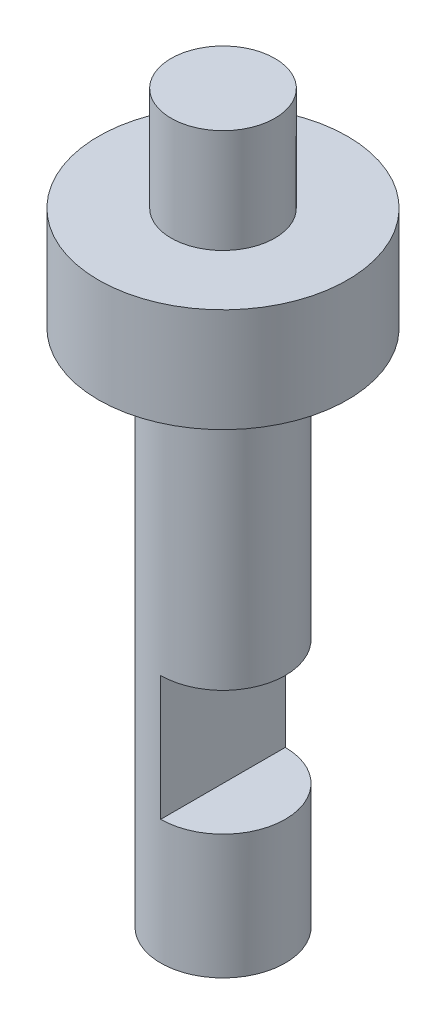
SolidWorks part; units mm, degrees
material "Plain Carbon Steel"
ref_plane "Front Plane" through (0, 0, 0) normal (0, 0, 1) x (1, 0, 0)
ref_plane "Top Plane" through (0, 0, 0) normal (0, 1, 0) x (1, 0, 0)
ref_plane "Right Plane" through (0, 0, 0) normal (1, 0, 0) x (0, 0, -1)
sketch "Pin Profile Sketch" plane through (0, 0, 0) normal (0, 0, 1) x (1, 0, 0)
  line L0 (0, 0) -> (-2.5, 0)
  line L1 (-2.5, 0) -> (-2.5, -5)
  line L2 (-2.5, -5) -> (-6, -5)
  line L3 (-6, -5) -> (-6, -10)
  line L4 (-6, -10) -> (-3, -10)
  line L5 (-3, -10) -> (-3, -35)
  line L6 (-3, -35) -> (0, -35)
  line L7 (0, -35) -> (0, 0)
  dimension "D1" = 2.5
  dimension "D2" = 6
  dimension "D3" = 3
  dimension "D4" = 5
  dimension "D5" = 5
  dimension "D6" = 25
revolve "Pin Body" add sketch "Pin Profile Sketch" angle 360 about L7
sketch "Side Notch Sketch" plane through (0, 0, 0) normal (0, 0, 1) x (1, 0, 0)
  line L0 (-3, -35) -> (3, -35) construction
  line L1 (0, -23) -> (8.5274, -23)
  line L2 (0, -23) -> (0, -29)
  line L3 (0, -29) -> (8.5274, -29)
  line L4 (8.5274, -23) -> (8.5274, -29)
  dimension "D1" = 6
  dimension "D2" = 6
  dimension "D3" = 8.5274
extrude "Side Notch 6x6" cut sketch "Side Notch Sketch" against normal mid plane 19
